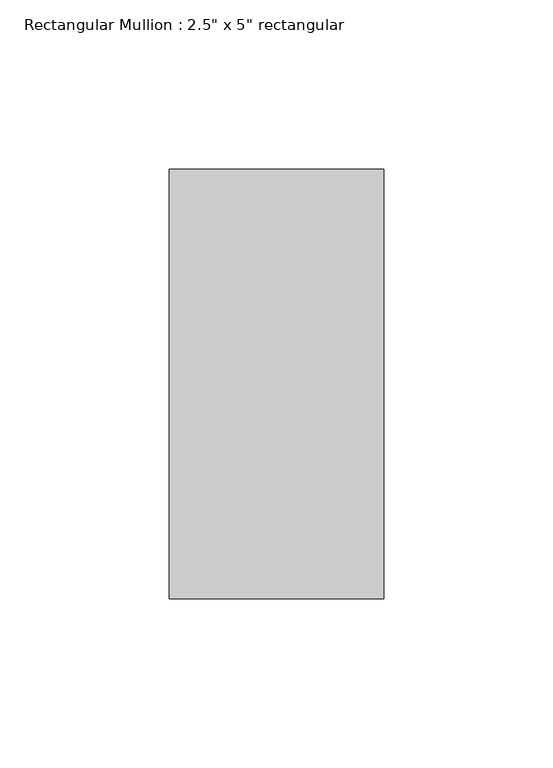
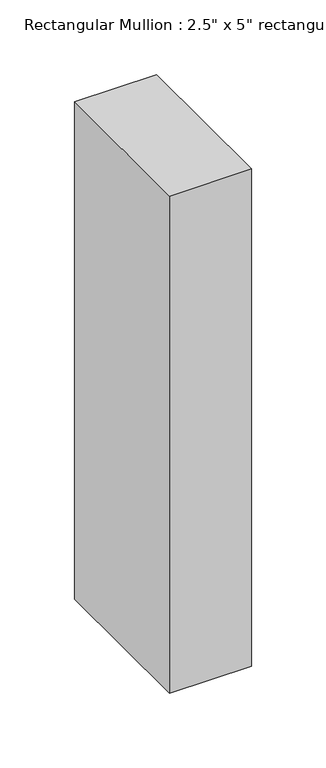
"""IFC4 building model written with IfcOpenShell, lengths in millimetres: member geometry."""

from ifc_helpers import new_model, si_unit, frame, origin, place, context, project, spatial, polyline, outline, extrude, source, transform, mapped, element, save


def member_7cfea1b5(model_context):
    return source(origin(), model_context, "Body", "SweptSolid", [
        extrude(outline(polyline([(0.0, 63.5), (0.0, -63.5), (-63.5, -63.5), (-63.5, 63.5), (0.0, 63.5)])), frame((0.0, 0.0, -406.4), z_axis=(0.0, 0.0, 1.0), x_axis=(1.0, 0.0, 0.0)), (0.0, 0.0, 1.0), 406.4),
    ])


if __name__ == "__main__":
    model = new_model("IFC4")
    model_context = context("Model", 3, world=origin())
    ifc_project = project(units=[si_unit("LENGTHUNIT", "METRE", prefix="MILLI")], contexts=[model_context])
    site = spatial("IfcSite", under=ifc_project)
    building = spatial("IfcBuilding", under=site)
    placement = place(None, origin())
    member_shape = member_7cfea1b5(model_context)
    element("IfcMember", 1, ObjectType="Rectangular Mullion : 2.5\" x 5\" rectangular", at=placement, inside=building, context=model_context, shape_type="MappedRepresentation", body=[
        mapped(member_shape, transform((0.0, 0.0, 0.0), x_axis=(1.0, 0.0, 0.0), y_axis=(0.0, 1.0, 0.0), z_axis=(0.0, 0.0, 1.0))),
    ])
    save(model, "model.ifc")

# Revit data of these elements
# Type "Rectangular Mullion : 2.5\" x 5\" rectangular"
#   built-in parameter 1007304 = 0.416667 (stored number, unit not read)
#   built-in parameter 1007301 = 0.104167 (stored number, unit not read)
#   built-in parameter 1007300 = 0.104167 (stored number, unit not read)
